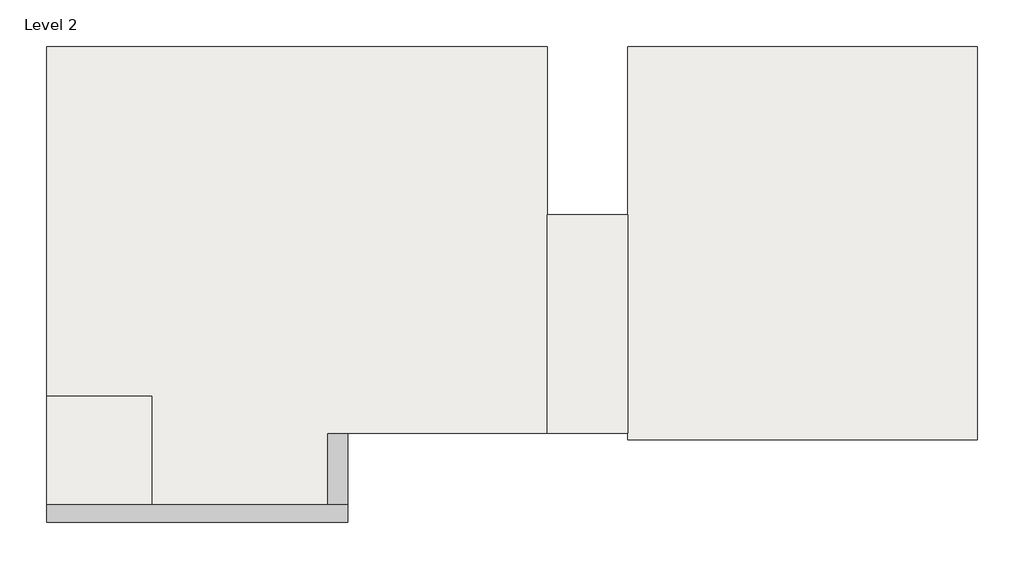
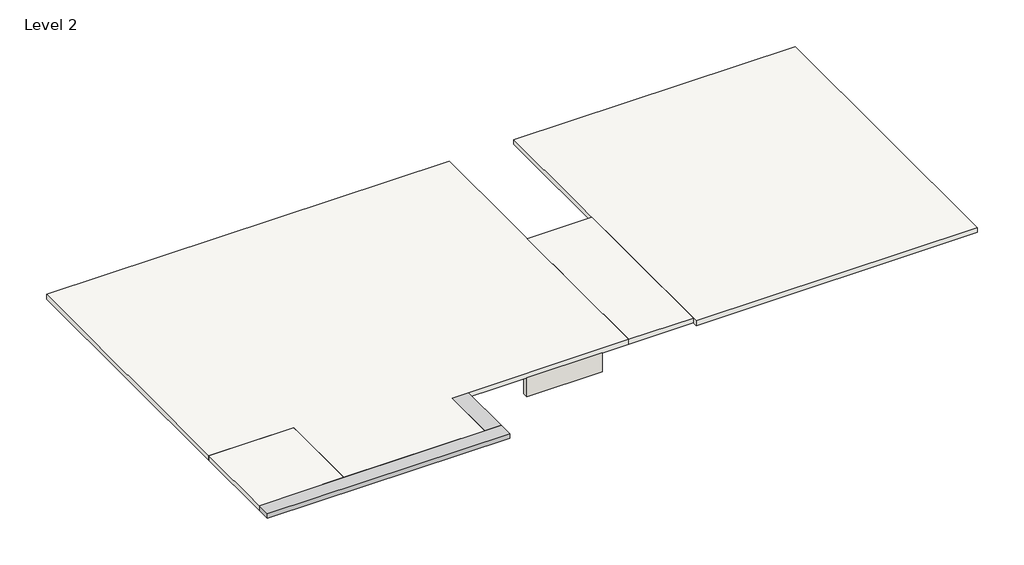
# One storey: 4 roofs, 1 proxy, 1 wall.
"""IFC4 building model written with IfcOpenShell, lengths in millimetres."""

from ifc_helpers import new_model, si_unit, frame, origin, place, context, project, spatial, polyline, outline, extrude, transform, mapped, element, save
from components import generic_models_15_generic_models_15_609883ec

model = new_model("IFC4")

# Units and contexts
model_context = context("Model", 3, world=origin())
ifc_project = project(units=[si_unit("LENGTHUNIT", "METRE", prefix="MILLI")], contexts=[model_context])

# Site, building, storey
site = spatial("IfcSite", under=ifc_project)
building = spatial("IfcBuilding", under=site)
storey = spatial("IfcBuildingStorey", under=building, Name="Level 2", Elevation=3048.0)

# Proxy
placement = place(None, origin())
generic_models_15_generic_models_15_shape = generic_models_15_generic_models_15_609883ec(model_context)
element("IfcBuildingElementProxy", 1, Name="Generic Models 15 : Generic Models 15", ObjectType="Generic Models 15 : Generic Models 15", at=placement, inside=storey, context=model_context, shape_type="MappedRepresentation", body=[
    mapped(generic_models_15_generic_models_15_shape, transform((0.0, 0.0, 0.0), x_axis=(1.0, 0.0, 0.0), y_axis=(0.0, 1.0, 0.0), z_axis=(0.0, 0.0, 1.0))),
])

# Roofs
element("IfcRoof", 2, ObjectType="6\"", at=placement, inside=storey, context=model_context, shape_type="SweptSolid", body=[
    extrude(outline(polyline([(-12100.1536806, -2804.7273102), (-12100.1536806, 5843.9726898), (282.3463194, 5843.9726898), (282.3463194, -3719.1273102), (-5165.9536806, -3719.1273102), (-5165.9536806, -5471.7273102), (-9495.3642415, -5471.7273102), (-9495.3642415, -2804.7273102), (-12100.1536806, -2804.7273102)])), frame((0.0, 0.0, 3048.0), z_axis=(0.0, 0.0, 1.0), x_axis=(1.0, 0.0, 0.0)), (0.0, 0.0, 1.0), 152.4),
])
element("IfcRoof", 3, ObjectType="6\"", at=placement, inside=storey, context=model_context, shape_type="SweptSolid", body=[
    extrude(outline(polyline([(2263.5463194, -3871.5273102), (2263.5463194, 5843.9726898), (10912.2463194, 5843.9726898), (10912.2463194, -3871.5273102), (2263.5463194, -3871.5273102)])), frame((0.0, 0.0, 3048.0), z_axis=(0.0, 0.0, 1.0), x_axis=(1.0, 0.0, 0.0)), (0.0, 0.0, 1.0), 152.4),
])
element("IfcRoof", 4, ObjectType="6\"", at=placement, inside=storey, context=model_context, shape_type="SweptSolid", body=[
    extrude(outline(polyline([(282.3463194, -3719.1273102), (282.3463194, 1691.0726898), (2263.5463194, 1691.0726898), (2263.5463194, -3719.1273102), (282.3463194, -3719.1273102)])), frame((0.0, 0.0, 3048.0), z_axis=(0.0, 0.0, 1.0), x_axis=(1.0, 0.0, 0.0)), (0.0, 0.0, 1.0), 152.4),
])
element("IfcRoof", 5, ObjectType="6\"", at=placement, inside=storey, context=model_context, shape_type="SweptSolid", body=[
    extrude(outline(polyline([(-12100.1536806, -2804.7273102), (-9495.3642415, -2804.7273102), (-9495.3642415, -5471.7273102), (-12100.1536806, -5471.7273102), (-12100.1536806, -2804.7273102)])), frame((0.0, 0.0, 3048.0), z_axis=(0.0, 0.0, 1.0), x_axis=(1.0, 0.0, 0.0)), (0.0, 0.0, 1.0), 152.4),
])

# Wall
element("IfcWall", 6, ObjectType="6\"", at=placement, inside=storey, context=model_context, shape_type="SweptSolid", body=[
    extrude(outline(polyline([(-530.4536806, -3719.1273102), (-2854.5536806, -3719.1273102), (-2854.5536806, -3566.7273102), (-530.4536806, -3566.7273102), (-530.4536806, -3719.1273102)])), frame((0.0, 0.0, 2438.4), z_axis=(0.0, 0.0, 1.0), x_axis=(1.0, 0.0, 0.0)), (0.0, 0.0, 1.0), 609.6),
])

save(model, "model.ifc")

# Revit data of these elements
# Type "6\""
#   Assembly Code = "B1020"
#   Layers, outside or top first: 0' - 6" no material (function 1)
# Type "6\""
#   Assembly Code = "B2010"
#   Layers, outside or top first: 0' - 6" "wall" (function 1)
# Element 1 (IfcBuildingElementProxy, "Generic Models 15 : Generic Models 15")
#   Phase Created = New Construction
#   Materials on its faces: "exterior wall", "wall"
# Elements 2, 3, 4 (IfcRoof, "6\"")
#   built-in parameter 1001705 = 10.5 (stored number, unit not read)
#   built-in parameter 1001710 = 33615
#   Phase Created = New Construction
#   Materials on its faces: "Default Roof"
# Element 5 (IfcRoof, "6\"")
#   built-in parameter 1001705 = 10.5 (stored number, unit not read)
#   built-in parameter 1001710 = 33615
#   Phase Created = New Construction
#   Materials on its faces: "Default Roof", "exterior wall"
# Element 6 (IfcWall, "6\"")
#   built-in parameter 1001111 = -2' - 0"
#   Top Offset = 0' - 0"
#   Base Offset = -2' - 0"
#   Unconnected Height = 2' - 0"
#   wall height = 2' - 0"
#   Phase Created = New Construction
#   Base Constraint = Level 2
#   Materials on its faces: "wall"
# Materials
#   "wall": class "Generic", colour RGB 127 127 127, transparency 0, Cost = 0
#   "exterior wall": class "Generic", colour RGB 215 217 121, transparency 0, Cost = 0
#   "Default Roof": colour RGB 88 101 114, transparency 0, Cost = 0
